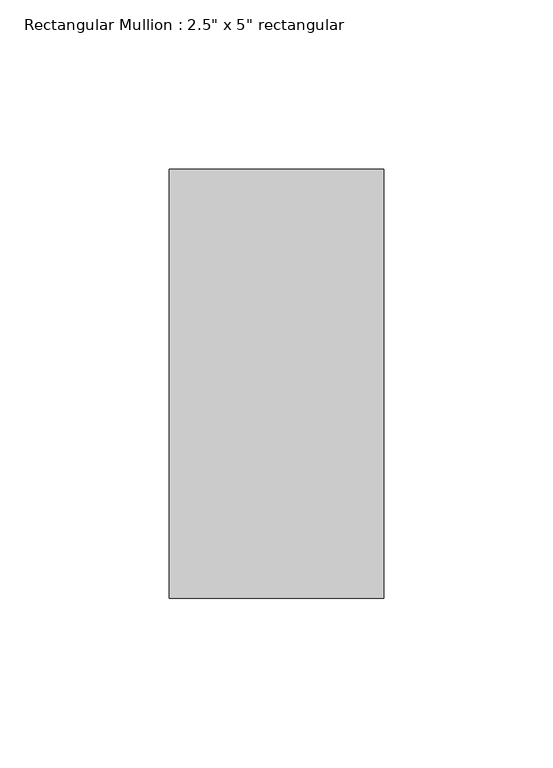
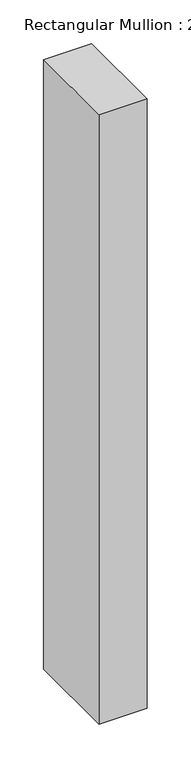
"""IFC4 building model written with IfcOpenShell, lengths in millimetres: member geometry."""

from ifc_helpers import new_model, si_unit, frame, origin, place, context, project, spatial, polyline, outline, extrude, source, transform, mapped, element, save


def member_7db1855a(model_context):
    return source(origin(), model_context, "Body", "SweptSolid", [
        extrude(outline(polyline([(31.75, 63.5), (31.75, -63.5), (-31.75, -63.5), (-31.75, 63.5), (31.75, 63.5)])), frame((0.0, 0.0, -850.9), z_axis=(0.0, 0.0, 1.0), x_axis=(1.0, 0.0, 0.0)), (0.0, 0.0, 1.0), 850.9),
    ])


if __name__ == "__main__":
    model = new_model("IFC4")
    model_context = context("Model", 3, world=origin())
    ifc_project = project(units=[si_unit("LENGTHUNIT", "METRE", prefix="MILLI")], contexts=[model_context])
    site = spatial("IfcSite", under=ifc_project)
    building = spatial("IfcBuilding", under=site)
    placement = place(None, origin())
    member_shape = member_7db1855a(model_context)
    element("IfcMember", 1, ObjectType="Rectangular Mullion : 2.5\" x 5\" rectangular", at=placement, inside=building, context=model_context, shape_type="MappedRepresentation", body=[
        mapped(member_shape, transform((0.0, 0.0, 0.0), x_axis=(1.0, 0.0, 0.0), y_axis=(0.0, 1.0, 0.0), z_axis=(0.0, 0.0, 1.0))),
    ])
    save(model, "model.ifc")

# Revit data of these elements
# Type "Rectangular Mullion : 2.5\" x 5\" rectangular"
#   built-in parameter 1007304 = 0.416667 (stored number, unit not read)
#   built-in parameter 1007301 = 0.104167 (stored number, unit not read)
#   built-in parameter 1007300 = 0.104167 (stored number, unit not read)
# Element 1 (IfcMember, "Rectangular Mullion : 2.5\" x 5\" rectangular")
#   Materials on its faces: "Iron, Ductile"
# Materials
#   "Iron, Ductile": class "Metal", colour RGB 0 0 0, transparency 0, Description = "Ductile cast iron", Cost = 0
